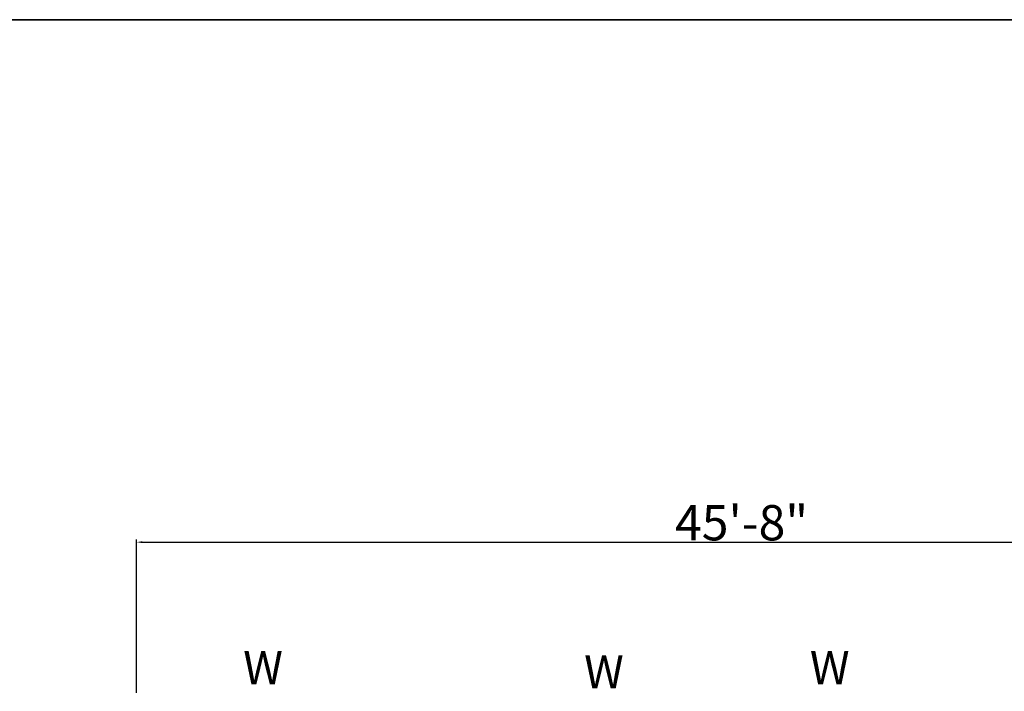
# Model space of a CAD drawing. Units: inches. Extents: x -31485 to -28799, y 18003 to 19130.
# Tile 14 of 15: x -29717 to -29271, y 18825 to 19130. Entities that reach past the tile are written whole.
import ezdxf

# ---------------------------------------------------------------- set-up
doc = ezdxf.new("R2010")
doc.units = ezdxf.units.IN
for name, color, linetype, lineweight in [('A-ANNO-DIMS', 2, 'Continuous', 18), ('A-ANNO-TEXT', 7, 'Continuous', 18), ('A-ANNO-TTLB', 7, 'Continuous', 35)]:
    doc.layers.add(name, color=color, linetype=linetype, lineweight=lineweight)
doc.styles.get("Standard").update_dxf_attribs({"font": 'arial.ttf'})
doc.dimstyles.new('ISO-25', dxfattribs={"dimtxt": 2.5, "dimasz": 2.5, "dimexe": 1.25, "dimexo": 0.625, "dimtad": 1, "dimdec": 0, "dimlunit": 3, "dimtxsty": 'Standard', "dimcen": 2.5, "dimadec": 0, "dimazin": 0, "dimtfac": 1, "dimtdec": 0, "dimtmove": 0, "dimatfit": 3, "dimfxl": 1, "dimarcsym": 0})

# ---------------------------------------------------------------- blocks, each defined once
blk = doc.blocks.new('*D204')
at = {"layer": 'A-ANNO-DIMS', "color": 0, "lineweight": -2, "transparency": 16777216}
for p, q in [((-29663.82, 18824.74), (-29663.82, 18894.35)), ((-29661.32, 18893.1), (-29118.32, 18893.1)), ((-29115.82, 18824.74), (-29115.82, 18894.35))]:
    blk.add_line(p, q, dxfattribs=at)
at = {"layer": 'A-ANNO-DIMS', "color": 0, "transparency": 16777216}
for points in [[(-29661.32, 18893.52), (-29661.32, 18892.68), (-29663.82, 18893.1)], [(-29118.32, 18893.52), (-29118.32, 18892.68), (-29115.82, 18893.1)]]:
    blk.add_solid(points, dxfattribs=at)
at = {"layer": 'Defpoints', "color": 0, "transparency": 16777216}
for p in [(-29115.82, 18893.1), (-29663.82, 18824.12), (-29115.82, 18824.12)]:
    blk.add_point(p, dxfattribs=at)
at = {"layer": 'A-ANNO-DIMS', "color": 0, "transparency": 16777216, "insert": (-29389.82, 18901.9), "char_height": 2.5, "attachment_point": 5}
blk.add_mtext('{\\H6.4x;45\'-8"}', dxfattribs=at)

msp = doc.modelspace()

# ---------------------------------------------------------------- linework, layer by layer
at = {"layer": 'A-ANNO-TTLB'}
msp.add_lwpolyline([(-31485.1, 19129.94), (-28798.64, 19129.94), (-28798.64, 18002.86), (-31485.1, 18002.86)], close=True, dxfattribs=at)

# ---------------------------------------------------------------- texts
at = {"layer": 'A-ANNO-TEXT', "char_height": 15, "attachment_point": 1}
for insert in [(-29615.55, 18843.69), (-29358.88, 18843.69), (-29461.14, 18841.84)]:
    msp.add_mtext_dynamic_manual_height_columns('{W}', width=1534.0875, gutter_width=12.5, heights=[0], dxfattribs=dict(at, insert=insert))

# ---------------------------------------------------------------- dimensions: what is measured, and where the dimension line sits
at = {"layer": 'A-ANNO-DIMS'}
dim = msp.add_linear_dim(base=(-29115.82, 18893.1), p1=(-29663.82, 18824.12), p2=(-29115.82, 18824.12), text='{\\H6.4x;<>}', dimstyle='ISO-25', override={"dimclrd": 0, "dimclre": 0, "dimclrt": 0}, dxfattribs=at)
dim.commit()
dim.dimension.update_dxf_attribs({"geometry": '*D204', "text_midpoint": (-29389.82, 18901.9)})

doc.saveas('drawing.dxf')
